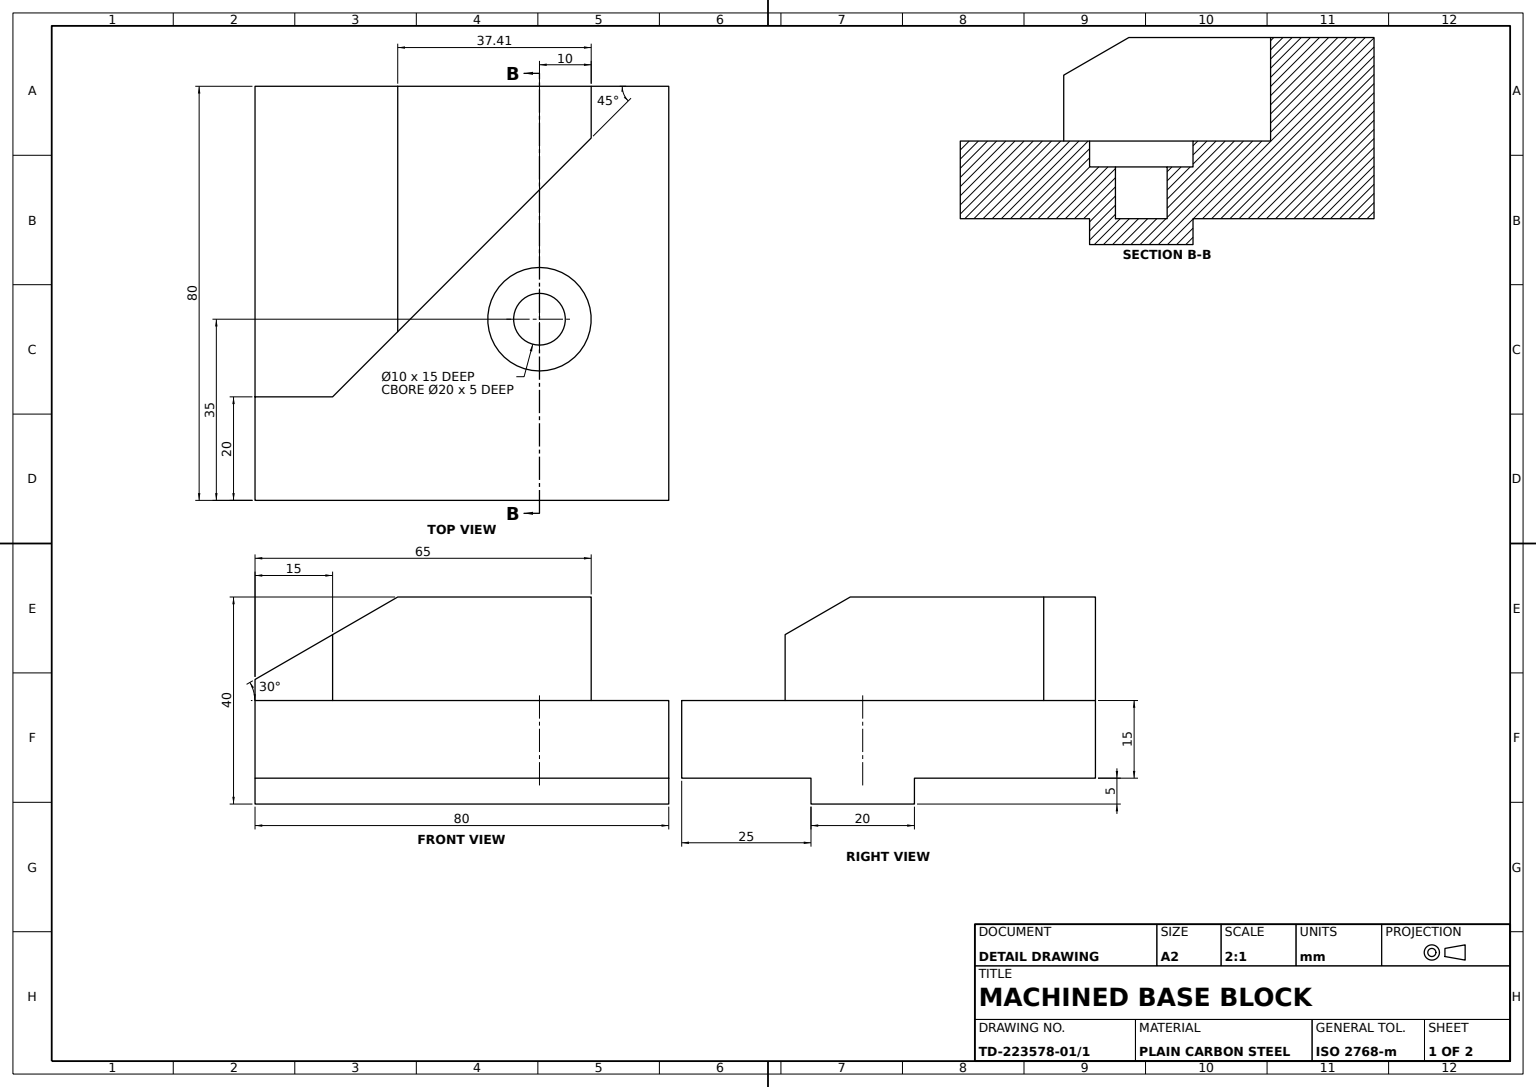
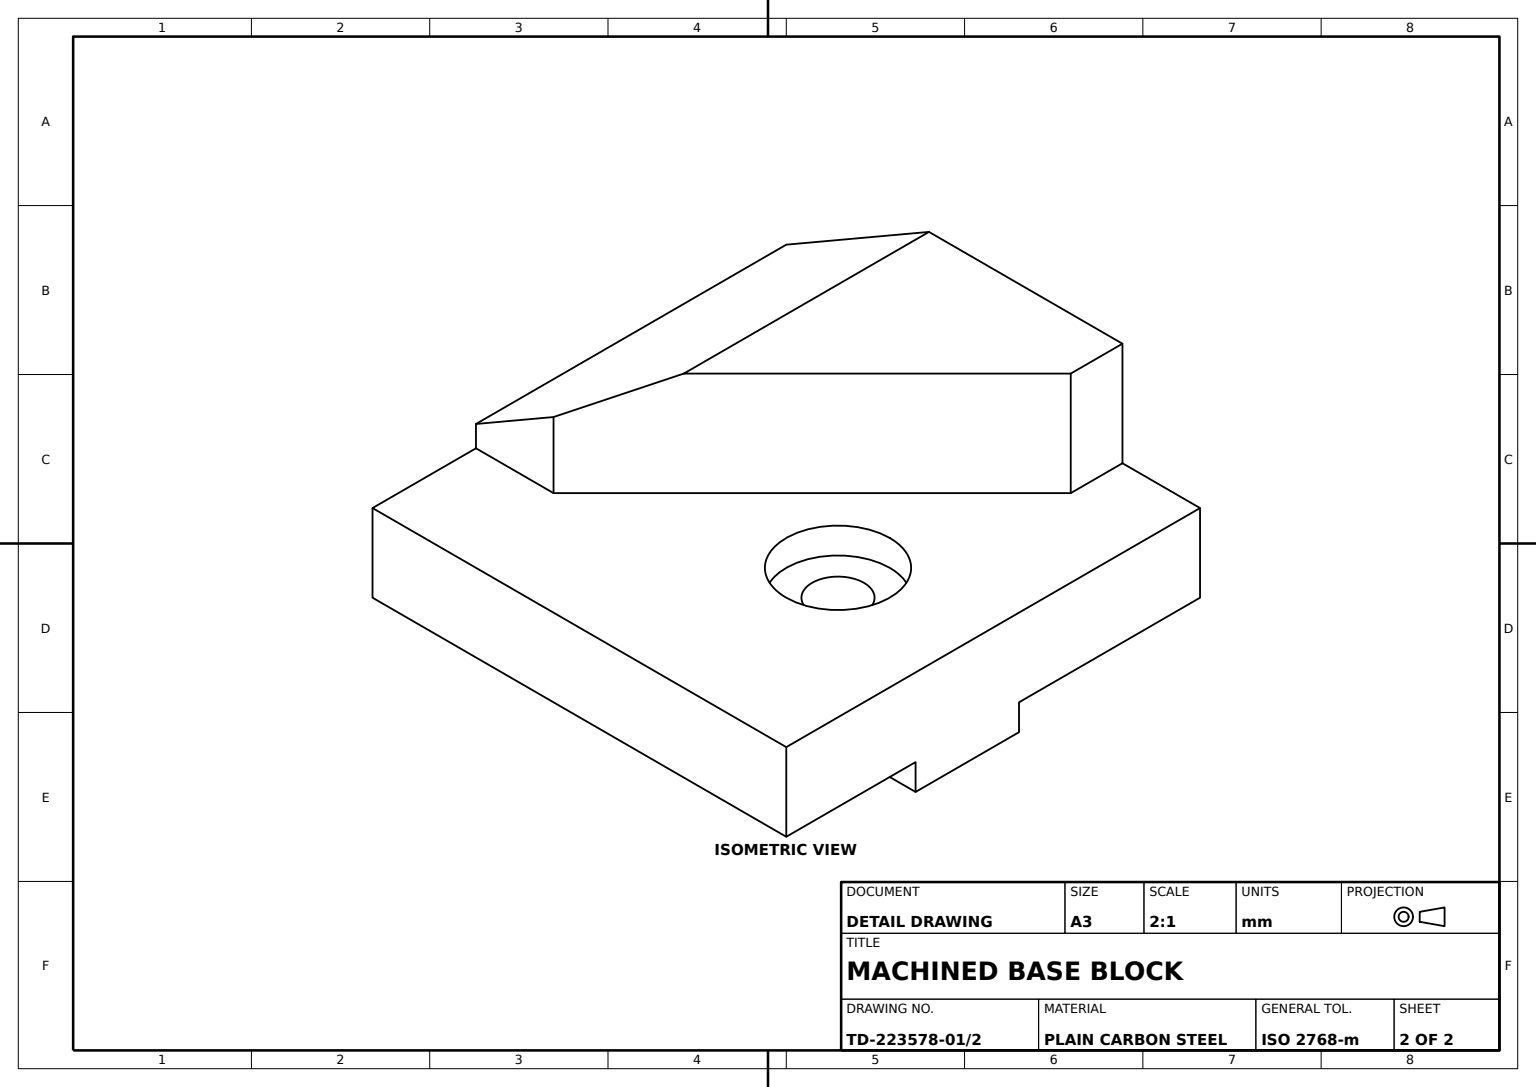
SolidWorks part; units mm, degrees
material "Plain Carbon Steel"
ref_plane "Front Plane" through (0, 0, 0) normal (0, 0, 1) x (1, 0, 0)
ref_plane "Top Plane" through (0, 0, 0) normal (0, 1, 0) x (1, 0, 0)
ref_plane "Right Plane" through (0, 0, 0) normal (1, 0, 0) x (0, 0, -1)
sketch "Base Plate Sketch" plane through (0, 0, 0) normal (0, 1, 0) x (1, 0, 0)
  line L0 (-34.7602, 45.2398) -> (45.2398, 45.2398)
  line L1 (45.2398, 45.2398) -> (45.2398, -34.7602)
  line L2 (45.2398, -34.7602) -> (-34.7602, -34.7602)
  line L3 (-34.7602, -34.7602) -> (-34.7602, 45.2398)
  line L4 (-34.7602, 45.2398) -> (45.2398, -34.7602) construction
  line L5 (-34.7602, -34.7602) -> (45.2398, 45.2398) construction
  dimension "D1" = 80
  dimension "D2" = 80
  dimension "D3" = 34.7602
extrude "Base Plate 80x80x20" add sketch "Base Plate Sketch" along normal blind 20
sketch "Bottom Slot Sketch" plane through (45.2398, 0, 0) normal (1, 0, 0) x (0, 0, -1)
  line L0 (-34.7602, 0) -> (-9.7602, 0)
  line L1 (-34.7602, 0) -> (45.2398, 0) construction
  line L2 (-9.7602, 0) -> (-9.7602, 5)
  line L3 (-9.7602, 5) -> (-34.7602, 5)
  line L4 (-34.7602, 20) -> (-34.7602, 0) construction
  line L5 (-34.7602, 5) -> (-34.7602, 0)
  line L6 (45.2398, 5) -> (10.2398, 5)
  line L7 (45.2398, 20) -> (45.2398, 0) construction
  line L8 (10.2398, 5) -> (10.2398, 0)
  line L9 (10.2398, 0) -> (45.2398, 0)
  line L10 (45.2398, 5) -> (45.2398, 0)
  dimension "D1" = 5
  dimension "D2" = 25
  dimension "D3" = 5
  dimension "D4" = 20
extrude "Bottom Slot" cut sketch "Bottom Slot Sketch" against normal blind 80
sketch "Raised Block Sketch" plane through (0, 20, 0) normal (0, 1, 0) x (1, 0, 0)
  line L0 (45.2398, 45.2398) -> (45.2398, -14.7602)
  line L1 (45.2398, -34.7602) -> (45.2398, 45.2398) construction
  line L2 (45.2398, -14.7602) -> (-34.7602, -14.7602)
  line L3 (-34.7602, 45.2398) -> (-34.7602, -34.7602) construction
  line L4 (-34.7602, -14.7602) -> (-34.7602, 45.2398)
  line L5 (-34.7602, 45.2398) -> (45.2398, 45.2398)
  line L6 (-34.7602, -34.7602) -> (45.2398, -34.7602) construction
  dimension "D1" = 20
extrude "Raised Block" add sketch "Raised Block Sketch" along normal blind 20
sketch "Block Step Cut 1 Sketch" plane through (0, 40, 0) normal (0, 1, 0) x (1, 0, 0)
  line L0 (45.2398, 45.2398) -> (45.2398, 35.2398)
  line L1 (45.2398, -14.7602) -> (45.2398, 45.2398) construction
  line L2 (45.2398, 35.2398) -> (30.2398, 35.2398)
  line L3 (30.2398, 35.2398) -> (30.2398, 45.2398)
  line L4 (45.2398, 45.2398) -> (-34.7602, 45.2398) construction
  line L5 (30.2398, 45.2398) -> (45.2398, 45.2398)
  dimension "D1" = 10
  dimension "D2" = 15
extrude "Block Step Cut 1" cut sketch "Block Step Cut 1 Sketch" against normal blind 20
sketch "Block Step Cut 2 Sketch" plane through (0, 40, 0) normal (0, 1, 0) x (1, 0, 0)
  line L0 (30.2398, 35.2398) -> (-19.7602, -14.7602)
  line L1 (30.2398, 35.2398) -> (45.2398, 35.2398)
  line L2 (45.2398, 35.2398) -> (45.2398, -14.7602)
  line L3 (45.2398, -14.7602) -> (-19.7602, -14.7602)
  dimension "D1" = 15
extrude "Block Step Cut 2" cut sketch "Block Step Cut 2 Sketch" against normal blind 20
sketch "Block Angle Cut 30deg Sketch" plane through (0, 0, -45.2398) normal (0, 0, -1) x (-1, 0, 0)
  line L0 (34.7602, 40) -> (7.168, 40)
  line L1 (-30.2398, 40) -> (34.7602, 40) construction
  line L2 (7.168, 40) -> (34.7602, 24.0696)
  line L3 (34.7602, 40) -> (34.7602, 24.0696)
  line L4 (-30.2398, 20) -> (-30.2398, 40) construction
  dimension "D1" = 30
  dimension "D2" = 37.4078
extrude "Block Angle Cut 30deg" cut sketch "Block Angle Cut 30deg Sketch" against normal up to next
sketch "Counterbore Ø25 Sketch" plane through (0, 20, 0) normal (0, 1, 0) x (1, 0, 0)
  line L0 (45.2398, -34.7602) -> (45.2398, 45.2398) construction
  line L1 (-34.7602, -34.7602) -> (45.2398, -34.7602) construction
  circle A0 centre (20.2398, 0.2398) radius 10
  dimension "D3" = 20
  dimension "D1" = 25
  dimension "D2" = 35
extrude "Counterbore Ø25x5" cut sketch "Counterbore Ø25 Sketch" against normal blind 5
sketch "Hole Ø10 Sketch" plane through (0, 15, 0) normal (0, 1, 0) x (1, 0, 0)
  circle A0 centre (20.2398, 0.2398) radius 5
  dimension "D1" = 10
extrude "Hole Ø10x10" cut sketch "Hole Ø10 Sketch" against normal blind 10
sketch "Auxiliary Body Profile Sketch" plane through (0, 0, 0) normal (0, 0, 1) x (1, 0, 0)
  line L0 (417.5031, -16.7661) -> (417.5031, -472.5945)
  line L18 (417.5031, -472.5945) -> (451.565, -472.5945)
  line L23 (451.565, -472.5945) -> (451.565, -269.4536)
  line L24 (451.565, -16.7661) -> (417.5031, -16.7661)
  line L25 (451.565, -227.1484) -> (635.9, -16.7661)
  line L27 (635.9, -16.7661) -> (672.9674, -16.7661)
  line L28 (672.9674, -16.7661) -> (519.8706, -191.4961)
  line L31 (494.6574, -220.2721) -> (589.8163, -472.5945)
  line L32 (589.8163, -472.5945) -> (625.8818, -472.5945)
  line L33 (625.8818, -472.5945) -> (519.8706, -191.4961)
  line L35 (451.565, -227.1484) -> (451.565, -16.7661)
  line L36 (494.6574, -220.2721) -> (451.565, -269.4536)
  point P16 (722.6616, -244.6803)
  point P20 (870.8066, -34.0781)
  point P25 (855.6994, -253.1679)
  point P29 (870.8066, -456.6271)
  dimension "D1" = 417.5031
  dimension "D2" = 16.7661
  dimension "D3" = 34.0619
  dimension "D4" = 455.8284
  dimension "D5" = 210.3823
  dimension "D6" = 279.7143
  dimension "D7" = 37.0674
  dimension "D8" = 65.3894
  dimension "D9" = 232.3127
  dimension "D10" = 269.6698
  dimension "D11" = 722.6616
  dimension "D12" = 244.6803
  dimension "D13" = 855.6994
  dimension "D14" = 253.1679
  dimension "D15" = 870.8066
  dimension "D16" = 34.0781
  dimension "D17" = 456.6271
extrude "Auxiliary Body Extrude" add sketch "Auxiliary Body Profile Sketch" along normal mid plane 100 separate body
fillet "Auxiliary Body Fillet R20" radius 20 3 edges at (519.8706, -191.4961, 0) (451.565, -269.4536, 0) (451.565, -227.1484, 0)
delete or keep bodies "Delete Auxiliary Body" type delete bodies bodies 110
